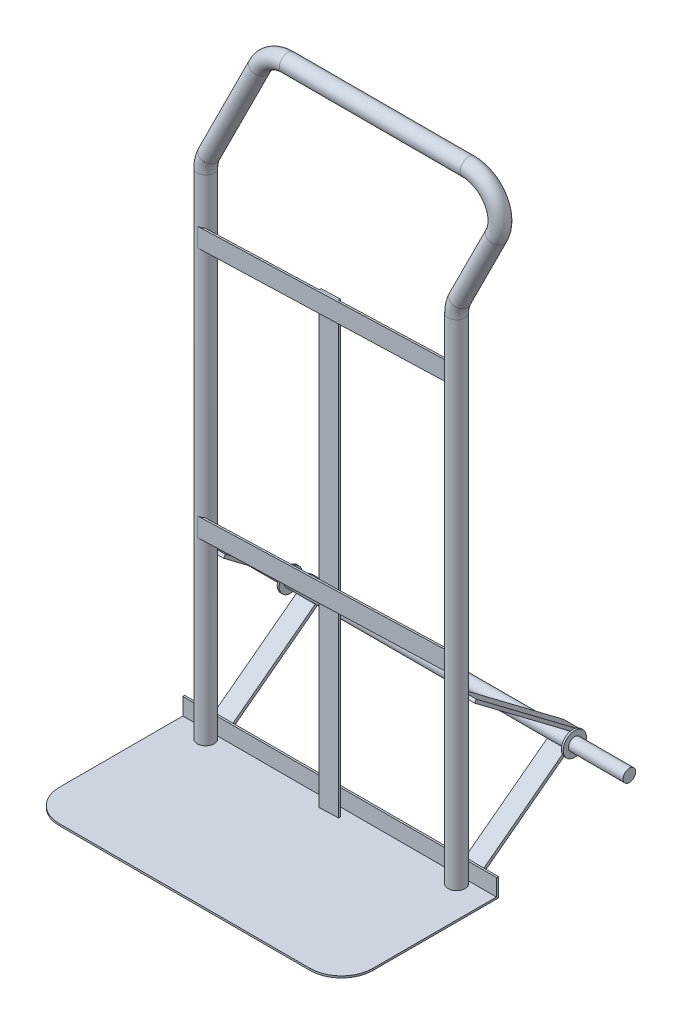
from build123d import *

# Parameters (mm, degrees)
SKETCH1_R                       = 13.45
SKETCH1_R_2                     = 10.25
PIPE_26_9_X_3_2_1_DEPTH         = 788.194321435
SKETCH1_ON_SEGMENT_2_R          = 13.45
SKETCH1_ON_SEGMENT_2_R_2        = 10.25
PIPE_26_9_X_3_2_1_2_ANGLE       = 26.57
SKETCH1_ON_SEGMENT_3_R          = 13.45
SKETCH1_ON_SEGMENT_3_R_2        = 10.25
PIPE_26_9_X_3_2_1_3_DEPTH       = 130.884808917
SKETCH1_ON_SEGMENT_4_R          = 13.45
SKETCH1_ON_SEGMENT_4_R_2        = 10.25
PIPE_26_9_X_3_2_1_4_ANGLE       = 116.57
SKETCH1_ON_SEGMENT_5_R          = 13.45
SKETCH1_ON_SEGMENT_5_R_2        = 10.25
PIPE_26_9_X_3_2_1_5_DEPTH       = 288.191772088
SKETCH1_ON_SEGMENT_6_R          = 13.45
SKETCH1_ON_SEGMENT_6_R_2        = 10.25
PIPE_26_9_X_3_2_1_6_ANGLE       = 63.43
SKETCH1_ON_SEGMENT_7_R          = 13.45
SKETCH1_ON_SEGMENT_7_R_2        = 10.25
PIPE_26_9_X_3_2_1_7_DEPTH       = 180.89560604
SKETCH1_ON_SEGMENT_8_R          = 13.45
SKETCH1_ON_SEGMENT_8_R_2        = 10.25
PIPE_26_9_X_3_2_1_8_ANGLE       = 26.57
SKETCH1_ON_SEGMENT_9_R          = 13.45
SKETCH1_ON_SEGMENT_9_R_2        = 10.25
PIPE_26_9_X_3_2_1_9_DEPTH       = 788.194321435
CROSS_BARS_SKETCH_W             = 400
CROSS_BARS_SKETCH_H             = 30
CROSS_BARS_30X3_DEPTH           = 3
CROSS_BARS_30X3_2_DEPTH         = 3
CENTRE_UPRIGHT_SKETCH_W         = 30
CENTRE_UPRIGHT_SKETCH_H         = 715
CENTRE_UPRIGHT_BAR_30X3_DEPTH   = 3
NOSE_PLATE_DEPTH                = 250
NOSE_PLATE_CORNER_FILLETS_R50_R = 50
AXLE_SKETCH_20_R                = 10
AXLE_20_DEPTH                   = 315
AXLE_BRACKET_DEPTH              = 15
WHEEL_COLLAR_SKETCH_37_R        = 18.5
WHEEL_COLLAR_37_DEPTH           = 3


with BuildPart() as part:
    # Sketch1 → Pipe 26.9 X 3.2(1) (new body)
    with BuildSketch(Plane(origin=(0, 0, 0), x_dir=(1, 0, 0), z_dir=(0, 1, 0))):
        Circle(SKETCH1_R)
        Circle(SKETCH1_R_2, mode=Mode.SUBTRACT)
    extrude(amount=PIPE_26_9_X_3_2_1_DEPTH)


with BuildPart() as body_2:
    # Sketch1 on segment 2 (carried to the start of arc 2) → Pipe 26.9 X 3.2_1 2 (revolve)
    with BuildSketch(Plane(origin=(0, 788.194321435, 0), x_dir=(1, 0, 0), z_dir=(0, 1, 0))):
        Circle(SKETCH1_ON_SEGMENT_2_R)
        Circle(SKETCH1_ON_SEGMENT_2_R_2, mode=Mode.SUBTRACT)
    revolve(axis=Axis((50, 788.194321435, 0), (0, 0, -1)), revolution_arc=PIPE_26_9_X_3_2_1_2_ANGLE)


with BuildPart() as body_3:
    # Sketch1 on segment 3 (carried to segment 3) → Pipe 26.9 X 3.2_1 3 (new body)
    with BuildSketch(Plane(origin=(5.280571981, 810.558863856, 0), x_dir=(0.89438856, -0.447290848, 0), z_dir=(0.447290848, 0.89438856, 0))):
        Circle(SKETCH1_ON_SEGMENT_3_R)
        Circle(SKETCH1_ON_SEGMENT_3_R_2, mode=Mode.SUBTRACT)
    extrude(amount=PIPE_26_9_X_3_2_1_3_DEPTH)


with BuildPart() as body_4:
    # Sketch1 on segment 4 (carried to the start of arc 4) → Pipe 26.9 X 3.2_1 4 (revolve)
    with BuildSketch(Plane(origin=(63.824149207, 927.620739678, 0), x_dir=(0.89438856, -0.447290848, 0), z_dir=(0.447290848, 0.89438856, 0))):
        Circle(SKETCH1_ON_SEGMENT_4_R)
        Circle(SKETCH1_ON_SEGMENT_4_R_2, mode=Mode.SUBTRACT)
    revolve(axis=Axis((19.104721189, 949.985282099, 0), (0, 0, 1)), revolution_arc=PIPE_26_9_X_3_2_1_4_ANGLE)


with BuildPart() as body_5:
    # Sketch1 on segment 5 (carried to segment 5) → Pipe 26.9 X 3.2_1 5 (new body)
    with BuildSketch(Plane(origin=(19.104721189, 999.985282099, 0), x_dir=(0, 1, 0), z_dir=(-1, 0, 0))):
        Circle(SKETCH1_ON_SEGMENT_5_R)
        Circle(SKETCH1_ON_SEGMENT_5_R_2, mode=Mode.SUBTRACT)
    extrude(amount=PIPE_26_9_X_3_2_1_5_DEPTH)


with BuildPart() as body_6:
    # Sketch1 on segment 6 (carried to the start of arc 6) → Pipe 26.9 X 3.2_1 6 (revolve)
    with BuildSketch(Plane(origin=(-269.087050899, 999.985282099, 0), x_dir=(0, 1, 0), z_dir=(-1, 0, 0))):
        Circle(SKETCH1_ON_SEGMENT_6_R)
        Circle(SKETCH1_ON_SEGMENT_6_R_2, mode=Mode.SUBTRACT)
    revolve(axis=Axis((-269.087050899, 949.985282099, 0), (0, 0, 1)), revolution_arc=PIPE_26_9_X_3_2_1_6_ANGLE)


with BuildPart() as body_7:
    # Sketch1 on segment 7 (carried to segment 7) → Pipe 26.9 X 3.2_1 7 (new body)
    with BuildSketch(Plane(origin=(-313.806478917, 972.34982452, 0), x_dir=(-0.89438856, 0.447290848, 0), z_dir=(-0.447290848, -0.89438856, 0))):
        Circle(SKETCH1_ON_SEGMENT_7_R)
        Circle(SKETCH1_ON_SEGMENT_7_R_2, mode=Mode.SUBTRACT)
    extrude(amount=PIPE_26_9_X_3_2_1_7_DEPTH)


with BuildPart() as body_8:
    # Sketch1 on segment 8 (carried to the start of arc 8) → Pipe 26.9 X 3.2_1 8 (revolve)
    with BuildSketch(Plane(origin=(-394.719428019, 810.558863856, 0), x_dir=(-0.89438856, 0.447290848, 0), z_dir=(-0.447290848, -0.89438856, 0))):
        Circle(SKETCH1_ON_SEGMENT_8_R)
        Circle(SKETCH1_ON_SEGMENT_8_R_2, mode=Mode.SUBTRACT)
    revolve(axis=Axis((-350, 788.194321435, 0), (0, 0, 1)), revolution_arc=PIPE_26_9_X_3_2_1_8_ANGLE)


with BuildPart() as body_9:
    # Sketch1 on segment 9 (carried to segment 9) → Pipe 26.9 X 3.2_1 9 (new body)
    with BuildSketch(Plane(origin=(-400, 0, 0), x_dir=(1, 0, 0), z_dir=(0, 1, 0))):
        Circle(SKETCH1_ON_SEGMENT_9_R)
        Circle(SKETCH1_ON_SEGMENT_9_R_2, mode=Mode.SUBTRACT)
    extrude(amount=PIPE_26_9_X_3_2_1_9_DEPTH)


with BuildPart() as body_10:
    # Cross Bars Sketch → Cross Bars 30x3 (new body)
    with BuildSketch(Plane(origin=(0, 0, 0), x_dir=(0.9994345198035738, 0, -0.03362500000000007), z_dir=(0.03362500000000007, 0, 0.9994345198035738))):
        with Locations((-199.886903961, 700)):
            Rectangle(CROSS_BARS_SKETCH_W, CROSS_BARS_SKETCH_H)
    extrude(amount=-CROSS_BARS_30X3_DEPTH)


with BuildPart() as body_11:
    # Cross Bars Sketch → Cross Bars 30x3 2 (new body)
    with BuildSketch(Plane(origin=(0, 0, 0), x_dir=(0.9994345198035738, 0, -0.03362500000000007), z_dir=(0.03362500000000007, 0, 0.9994345198035738))):
        with Locations((-199.886903961, 300)):
            Rectangle(CROSS_BARS_SKETCH_W, CROSS_BARS_SKETCH_H)
    extrude(amount=-CROSS_BARS_30X3_2_DEPTH)


with BuildPart() as body_12:
    # Centre Upright Sketch → Centre Upright Bar 30x3 (new body)
    with BuildSketch(Plane(origin=(-0.100875, 0, -2.998303559), x_dir=(-0.9994345198035738, 0, 0.033625000000000065), z_dir=(-0.033625000000000065, 0, -0.9994345198035738))):
        with Locations((199.886903961, 357.5)):
            Rectangle(CENTRE_UPRIGHT_SKETCH_W, CENTRE_UPRIGHT_SKETCH_H)
    extrude(amount=CENTRE_UPRIGHT_BAR_30X3_DEPTH)


with BuildPart() as body_13:
    # Nose Plate Profile → Nose Plate (new, symmetric)
    with BuildSketch(Plane(origin=(-200, 0, 0), x_dir=(0, 0, -1), z_dir=(1, 0, 0))):
        Polygon((16.45, 27), (16.45, -3), (-233.55, -3), (-233.55, 0), (13.45, 0), (13.45, 27), align=None)
    extrude(amount=NOSE_PLATE_DEPTH, both=True)

    # Nose Plate Corner Fillets R50
    nose_plate_corner_fillets_r50_edges = [body_13.edges().sort_by_distance(p)[0] for p in [
        (50, -1.5, 233.55),
        (-450, -1.5, 233.55),
    ]]
    fillet(nose_plate_corner_fillets_r50_edges, radius=NOSE_PLATE_CORNER_FILLETS_R50_R)


with BuildPart() as body_14:
    # Axle Sketch Ø20 → Axle Ø20 (new, symmetric)
    with BuildSketch(Plane(origin=(-200, 0, 0), x_dir=(0, 0, -1), z_dir=(1, 0, 0))):
        with Locations((160.45, 127)):
            Circle(AXLE_SKETCH_20_R)
    extrude(amount=AXLE_20_DEPTH, both=True)


with BuildPart() as body_15:
    # Axle Bracket Profile → Axle Bracket (new, symmetric)
    with BuildSketch(Plane(origin=(0, 0, 0), x_dir=(0, 0, -1), z_dir=(1, 0, 0))):
        Polygon((177.066401411, 127), (13.45, 250.293801947), (16.459075116, 254.286979497), (185.374602117, 127), (16.459075116, -0.286979497), (13.45, 3.706198053), align=None)
    axle_bracket = extrude(amount=AXLE_BRACKET_DEPTH, both=True)


with BuildPart() as body_13_1:
    add(body_13.part)

    # Axle Bracket Mirror: Axle Bracket across plane
    add(axle_bracket.mirror(Plane(origin=(-200, 0, 0), x_dir=(0, 0, 1), z_dir=(1, 0, 0))))


with BuildPart() as body_16:
    # Wheel Collar Sketch Ø37 → Wheel Collar Ø37 (new body)
    with BuildSketch(Plane(origin=(25, 0, 0), x_dir=(0, 0, -1), z_dir=(1, 0, 0))):
        with Locations((160.45, 127)):
            Circle(WHEEL_COLLAR_SKETCH_37_R)
    wheel_collar_37 = extrude(amount=WHEEL_COLLAR_37_DEPTH)


with BuildPart() as body_14_1:
    add(body_14.part)

    # Wheel Collar Mirror: Wheel Collar Ø37 across plane
    add(wheel_collar_37.mirror(Plane(origin=(-200, 0, 0), x_dir=(0, 0, 1), z_dir=(1, 0, 0))))


solid = Compound([part.part, body_2.part, body_3.part, body_4.part, body_5.part, body_6.part, body_7.part, body_8.part, body_9.part, body_10.part, body_11.part, body_12.part, body_15.part, body_13_1.part, body_16.part, body_14_1.part])
